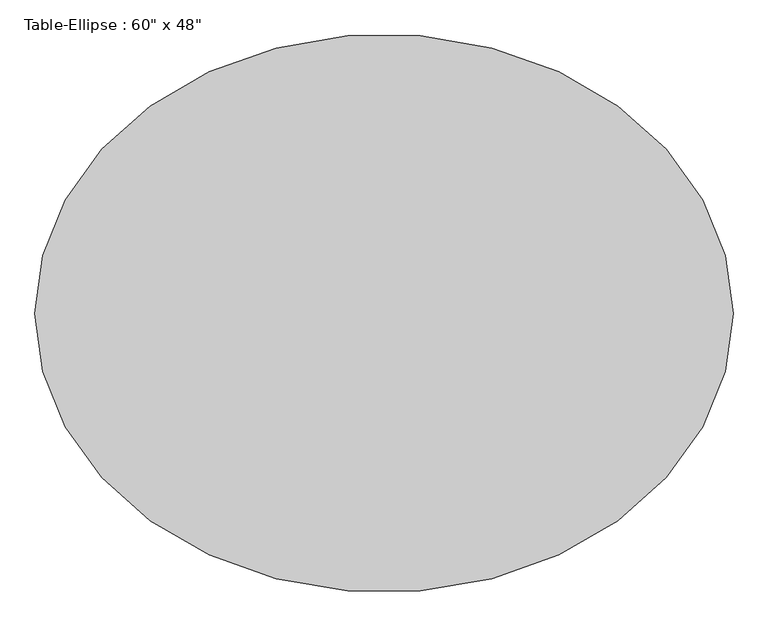
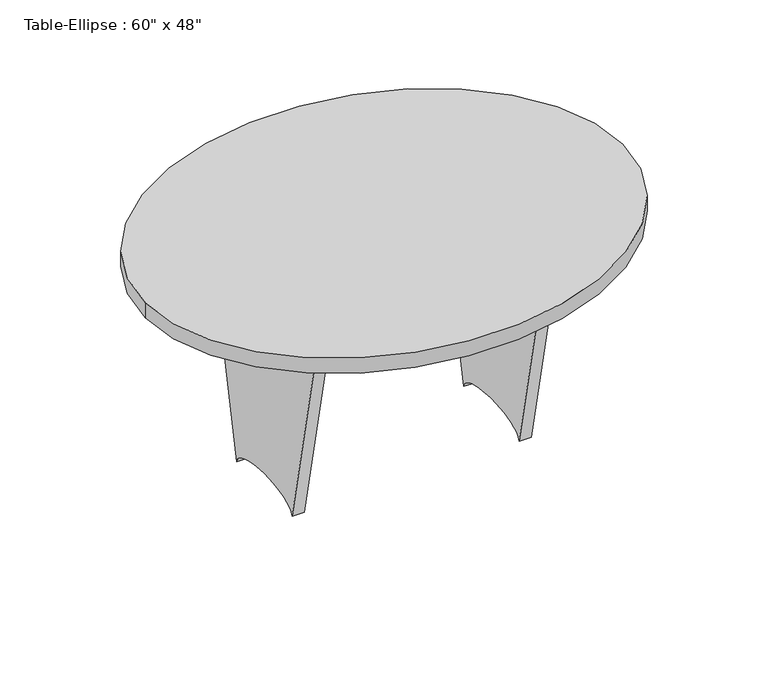
"""IFC4 building model written with IfcOpenShell, lengths in millimetres: furniture geometry."""

from ifc_helpers import new_model, si_unit, point, frame, origin, place, context, project, spatial, ellipse_curve, trimmed, source, transform, mapped, element, save
from ifc_brep_helpers import plane_surface, extruded_surface, advanced_brep


def furniture_743965d2(model_context):
    return source(origin(), model_context, "Body", "AdvancedBrep", [
        advanced_brep(
        [(-342.9, 19.05, 711.2), (342.9, 19.05, 711.2), (342.9, 19.05, 474.1333333), (-342.9, 19.05, 474.1333333), (-342.9, -19.05, 711.2), (-342.9, -19.05, 474.1333333), (342.9, -19.05, 474.1333333), (342.9, -19.05, 711.2)],
        [
            (0, 1),
            (1, 2),
            (2, 3, ellipse_curve(frame((0.0, 19.05, 474.1333333), z_axis=(0.0, -1.0, 0.0), x_axis=(1.0, 0.0, 0.0)), 342.9, 101.6)),
            (3, 0),
            (4, 5),
            (5, 6, ellipse_curve(frame((0.0, -19.05, 474.1333333), z_axis=(0.0, 1.0, 0.0), x_axis=(1.0, 0.0, 0.0)), 342.9, 101.6)),
            (6, 7),
            (7, 4),
            (0, 4),
            (7, 1),
            (6, 2),
            (5, 3),
        ],
        [
            plane_surface(frame((-342.9, 19.05, 711.2), z_axis=(0.0, 1.0, 0.0), x_axis=(1.0, 0.0, 0.0))),
            plane_surface(frame((-342.9, -19.05, 711.2), z_axis=(0.0, -1.0, 0.0), x_axis=(-1.0, 0.0, 0.0))),
            plane_surface(frame((-342.9, 19.05, 711.2), z_axis=(0.0, 0.0, 1.0), x_axis=(0.0, -1.0, 0.0))),
            plane_surface(frame((342.9, 19.05, 711.2), z_axis=(1.0, 0.0, 0.0), x_axis=(0.0, -1.0, 0.0))),
            extruded_surface(trimmed(ellipse_curve(frame((0.0, -57.15, 474.1333333), z_axis=(0.0, -1.0, 0.0), x_axis=(1.0, 0.0, 0.0)), 342.9, 101.6), [point((342.9, -57.15, 474.1333333))], [point((-342.9, -57.15, 474.1333333))], True, "CARTESIAN"), (0.0, 38.099999999999994, 0.0), 38.099999999999994),
            plane_surface(frame((-342.9, 19.05, 474.1333333), z_axis=(-1.0, 0.0, 0.0), x_axis=(0.0, -1.0, 0.0))),
        ],
        [
            (0, [[1, 2, 3, 4]]),
            (1, [[5, 6, 7, 8]]),
            (2, [[-1, 9, -8, 10]]),
            (3, [[-2, -10, -7, 11]]),
            (4, [[-3, -11, -6, 12]]),
            (5, [[-4, -12, -5, -9]]),
        ],
    ),
        advanced_brep(
        [(381.0, 304.8, 711.2), (381.0, -304.8, 711.2), (381.0, -152.4, 0.0), (381.0, 152.4, 0.0), (342.9, 304.8, 711.2), (342.9, 152.4, 0.0), (342.9, -152.4, 0.0), (342.9, -304.8, 711.2)],
        [
            (0, 1),
            (1, 2),
            (2, 3, ellipse_curve(frame((381.0, 0.0, 0.0), z_axis=(-1.0, 0.0, 0.0), x_axis=(0.0, 1.0, 0.0)), 152.4, 50.8)),
            (3, 0),
            (4, 5),
            (5, 6, ellipse_curve(frame((342.9, 0.0, 0.0), z_axis=(1.0, 0.0, 0.0), x_axis=(0.0, 1.0, 0.0)), 152.4, 50.8)),
            (6, 7),
            (7, 4),
            (0, 4),
            (7, 1),
            (6, 2),
            (5, 3),
        ],
        [
            plane_surface(frame((381.0, -304.8, 711.2), z_axis=(1.0, 0.0, 0.0), x_axis=(0.0, -1.0, 0.0))),
            plane_surface(frame((342.9, -304.8, 711.2), z_axis=(-1.0, 0.0, 0.0), x_axis=(0.0, 1.0, 0.0))),
            plane_surface(frame((381.0, 304.8, 711.2), z_axis=(0.0, 0.0, 1.0), x_axis=(-1.0, 0.0, 0.0))),
            plane_surface(frame((381.0, -304.8, 711.2), z_axis=(0.0, -0.9778024140774091, -0.2095290887308754), x_axis=(-1.0, 0.0, 0.0))),
            extruded_surface(trimmed(ellipse_curve(frame((304.8, 0.0, 0.0), z_axis=(-1.0, 0.0, 0.0), x_axis=(0.0, 1.0, 0.0)), 152.4, 50.8), [point((304.8, -152.4, 0.0))], [point((304.8, 152.4, 0.0))], True, "CARTESIAN"), (38.099999999999966, 0.0, 0.0), 38.099999999999966),
            plane_surface(frame((381.0, 152.4, 0.0), z_axis=(0.0, 0.977802414077412, -0.2095290887308621), x_axis=(-1.0, 0.0, 0.0))),
        ],
        [
            (0, [[1, 2, 3, 4]]),
            (1, [[5, 6, 7, 8]]),
            (2, [[-1, 9, -8, 10]]),
            (3, [[-2, -10, -7, 11]]),
            (4, [[-3, -11, -6, 12]]),
            (5, [[-4, -12, -5, -9]]),
        ],
    ),
        advanced_brep(
        [(-342.9, 304.8, 711.2), (-342.9, -304.8, 711.2), (-342.9, -152.4, 0.0), (-342.9, 152.4, 0.0), (-381.0, 304.8, 711.2), (-381.0, 152.4, 0.0), (-381.0, -152.4, 0.0), (-381.0, -304.8, 711.2)],
        [
            (0, 1),
            (1, 2),
            (2, 3, ellipse_curve(frame((-342.9, 0.0, 0.0), z_axis=(-1.0, 0.0, 0.0), x_axis=(0.0, 1.0, 0.0)), 152.4, 50.8)),
            (3, 0),
            (4, 5),
            (5, 6, ellipse_curve(frame((-381.0, 0.0, 0.0), z_axis=(1.0, 0.0, 0.0), x_axis=(0.0, 1.0, 0.0)), 152.4, 50.8)),
            (6, 7),
            (7, 4),
            (0, 4),
            (7, 1),
            (6, 2),
            (5, 3),
        ],
        [
            plane_surface(frame((-342.9, -304.8, 711.2), z_axis=(1.0, 0.0, 0.0), x_axis=(0.0, -1.0, 0.0))),
            plane_surface(frame((-381.0, -304.8, 711.2), z_axis=(-1.0, 0.0, 0.0), x_axis=(0.0, 1.0, 0.0))),
            plane_surface(frame((-342.9, 304.8, 711.2), z_axis=(0.0, 0.0, 1.0), x_axis=(-1.0, 0.0, 0.0))),
            plane_surface(frame((-342.9, -304.8, 711.2), z_axis=(0.0, -0.9778024140774088, -0.2095290887308767), x_axis=(-1.0, 0.0, 0.0))),
            extruded_surface(trimmed(ellipse_curve(frame((-419.1, 0.0, 0.0), z_axis=(-1.0, 0.0, 0.0), x_axis=(0.0, 1.0, 0.0)), 152.4, 50.8), [point((-419.1, -152.4, 0.0))], [point((-419.1, 152.4, 0.0))], True, "CARTESIAN"), (38.10000000000002, 0.0, 0.0), 38.10000000000002),
            plane_surface(frame((-342.9, 152.4, 0.0), z_axis=(0.0, 0.9778024140774109, -0.2095290887308677), x_axis=(-1.0, 0.0, 0.0))),
        ],
        [
            (0, [[1, 2, 3, 4]]),
            (1, [[5, 6, 7, 8]]),
            (2, [[-1, 9, -8, 10]]),
            (3, [[-2, -10, -7, 11]]),
            (4, [[-3, -11, -6, 12]]),
            (5, [[-4, -12, -5, -9]]),
        ],
    ),
        advanced_brep(
        [(-762.0, 0.0, 762.0), (762.0, 0.0, 762.0), (-762.0, 0.0, 711.2), (762.0, 0.0, 711.2)],
        [
            (0, 1, ellipse_curve(frame((0.0, 0.0, 762.0), z_axis=(0.0, 0.0, 1.0), x_axis=(1.0, 0.0, 0.0)), 762.0, 609.6)),
            (1, 0, ellipse_curve(frame((0.0, 0.0, 762.0), z_axis=(0.0, 0.0, 1.0), x_axis=(1.0, 0.0, 0.0)), 762.0, 609.6)),
            (2, 3, ellipse_curve(frame((0.0, 0.0, 711.2), z_axis=(0.0, 0.0, -1.0), x_axis=(1.0, 0.0, 0.0)), 762.0, 609.6)),
            (3, 2, ellipse_curve(frame((0.0, 0.0, 711.2), z_axis=(0.0, 0.0, -1.0), x_axis=(1.0, 0.0, 0.0)), 762.0, 609.6)),
            (0, 2),
            (3, 1),
        ],
        [
            plane_surface(frame((762.0, 0.0, 762.0), z_axis=(0.0, 0.0, 1.0), x_axis=(0.0, 1.0, 0.0))),
            plane_surface(frame((762.0, 0.0, 711.2), z_axis=(0.0, 0.0, -1.0), x_axis=(0.0, -1.0, 0.0))),
            extruded_surface(trimmed(ellipse_curve(frame((0.0, 0.0, 660.4), z_axis=(0.0, 0.0, 1.0), x_axis=(1.0, 0.0, 0.0)), 762.0, 609.6), [point((-762.0, 0.0, 660.4))], [point((762.0, 0.0, 660.4))], True, "CARTESIAN"), (0.0, 0.0, 50.80000000000007), 50.80000000000007),
            extruded_surface(trimmed(ellipse_curve(frame((0.0, 0.0, 660.4), z_axis=(0.0, 0.0, 1.0), x_axis=(1.0, 0.0, 0.0)), 762.0, 609.6), [point((762.0, 0.0, 660.4))], [point((-762.0, 0.0, 660.4))], True, "CARTESIAN"), (0.0, 0.0, 50.80000000000007), 50.80000000000007),
        ],
        [
            (0, [[1, 2]]),
            (1, [[3, 4]]),
            (2, [[-1, 5, -4, 6]]),
            (3, [[-2, -6, -3, -5]]),
        ],
    ),
    ])


if __name__ == "__main__":
    model = new_model("IFC4")
    model_context = context("Model", 3, world=origin())
    ifc_project = project(units=[si_unit("LENGTHUNIT", "METRE", prefix="MILLI")], contexts=[model_context])
    site = spatial("IfcSite", under=ifc_project)
    building = spatial("IfcBuilding", under=site)
    placement = place(None, origin())
    furniture_shape = furniture_743965d2(model_context)
    element("IfcFurniture", 1, ObjectType="Table-Ellipse : 60\" x 48\"", at=placement, inside=building, context=model_context, shape_type="MappedRepresentation", body=[
        mapped(furniture_shape, transform((0.0, 0.0, 0.0), x_axis=(1.0, 0.0, 0.0), y_axis=(0.0, 1.0, 0.0), z_axis=(0.0, 0.0, 1.0))),
    ])
    save(model, "model.ifc")

# Revit data of these elements
# Type "Table-Ellipse : 60\" x 48\""
#   Assembly Code = "E2020200"
#   Half Width = 2' - 0"
#   Half Length = 2' - 6"
#   Height = 2' - 6"
#   Length = 5' - 0"
#   Width = 4' - 0"
#   Base Material = Birch
#   Top Material = Birch
#   Default Elevation = 0
# Element 1 (IfcFurniture, "Table-Ellipse : 60\" x 48\"")
#   Materials on its faces: "Birch"
# Materials
#   "Birch": class "Wood", colour RGB 224 178 126, transparency 0, Description = "Betula Alleghaniensis", Cost = 0
